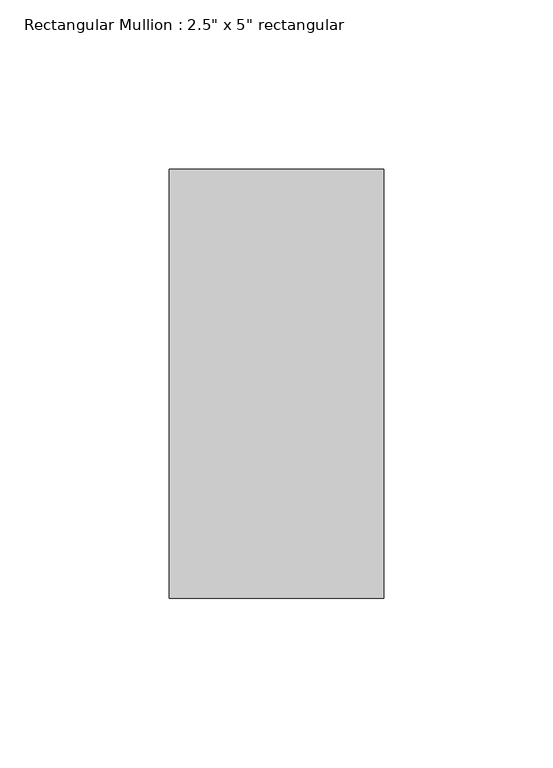
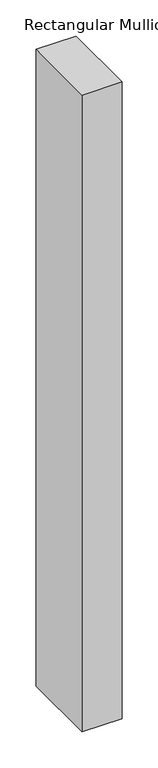
"""IFC4 building model written with IfcOpenShell, lengths in millimetres: member geometry."""

from ifc_helpers import new_model, si_unit, frame, origin, place, context, project, spatial, polyline, outline, extrude, source, transform, mapped, element, save


def member_4d6ef9b1(model_context):
    return source(origin(), model_context, "Body", "SweptSolid", [
        extrude(outline(polyline([(0.0, 63.5), (0.0, -63.5), (-63.5, -63.5), (-63.5, 63.5), (0.0, 63.5)])), frame((0.0, 0.0, -1073.15), z_axis=(0.0, 0.0, 1.0), x_axis=(1.0, 0.0, 0.0)), (0.0, 0.0, 1.0), 1073.15),
    ])


if __name__ == "__main__":
    model = new_model("IFC4")
    model_context = context("Model", 3, world=origin())
    ifc_project = project(units=[si_unit("LENGTHUNIT", "METRE", prefix="MILLI")], contexts=[model_context])
    site = spatial("IfcSite", under=ifc_project)
    building = spatial("IfcBuilding", under=site)
    placement = place(None, origin())
    member_shape = member_4d6ef9b1(model_context)
    element("IfcMember", 1, ObjectType="Rectangular Mullion : 2.5\" x 5\" rectangular", at=placement, inside=building, context=model_context, shape_type="MappedRepresentation", body=[
        mapped(member_shape, transform((0.0, 0.0, 0.0), x_axis=(1.0, 0.0, 0.0), y_axis=(0.0, 1.0, 0.0), z_axis=(0.0, 0.0, 1.0))),
    ])
    save(model, "model.ifc")

# Revit data of these elements
# Type "Rectangular Mullion : 2.5\" x 5\" rectangular"
#   built-in parameter 1007304 = 0.416667 (stored number, unit not read)
#   built-in parameter 1007301 = 0.104167 (stored number, unit not read)
#   built-in parameter 1007300 = 0.104167 (stored number, unit not read)
# Element 1 (IfcMember, "Rectangular Mullion : 2.5\" x 5\" rectangular")
#   Materials on its faces: "Aluminum"
# Materials
#   "Aluminum": class "Metal", colour RGB 247 247 247, transparency 0, Description = "Aluminum 6061", Cost = 0
